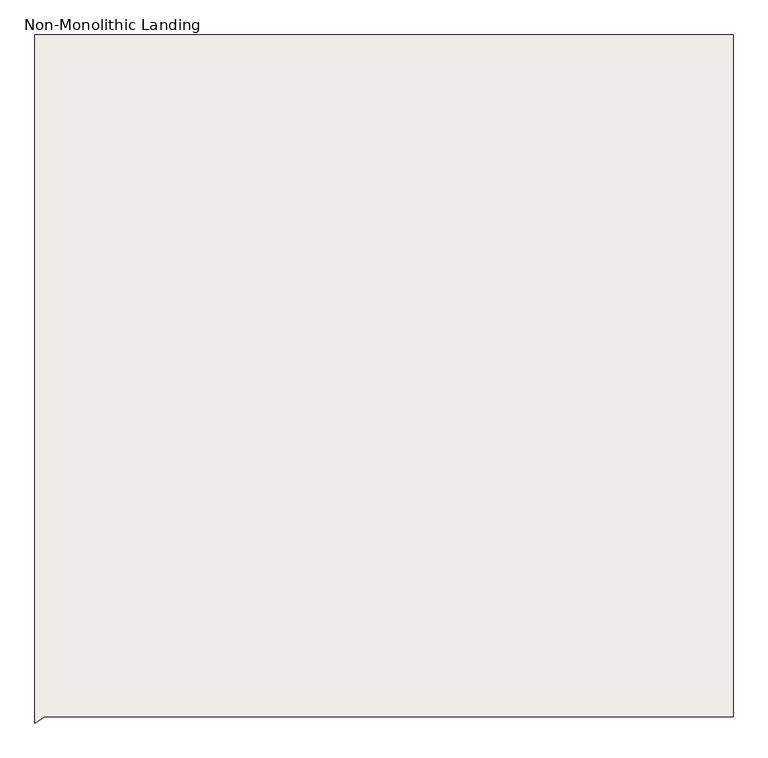
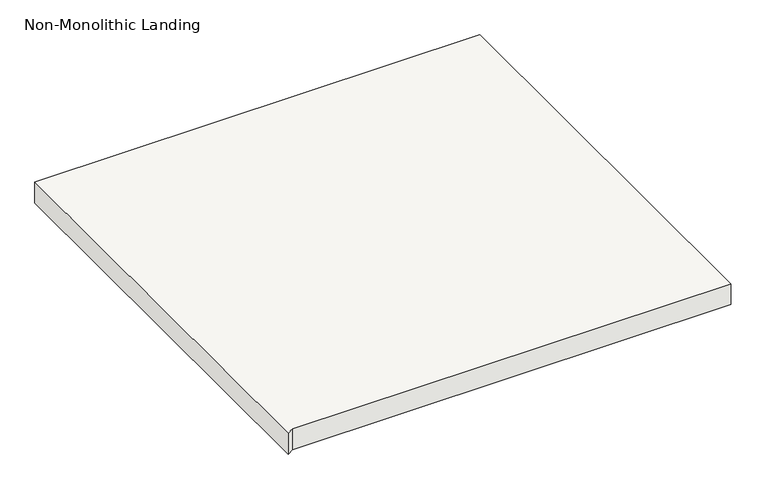
"""IFC4 building model written with IfcOpenShell, lengths in millimetres: slab geometry, Non-Monolithic Landing."""

from ifc_helpers import new_model, si_unit, frame, origin, place, context, project, spatial, polyline, outline, extrude, source, transform, mapped, element, save


def non_monolithic_landing_cef648f3(model_context):
    return source(origin(), model_context, "Body", "SweptSolid", [
        extrude(outline(polyline([(-10492.1794909, -1507.9618509), (-9477.5794909, -1507.9618509), (-9477.5794909, -2498.5618509), (-10477.6052721, -2498.5618509), (-10492.1794909, -2507.9876321), (-10492.1794909, -1507.9618509)])), frame((0.0, 0.0, 10869.0117647), z_axis=(0.0, 0.0, 1.0), x_axis=(1.0, 0.0, 0.0)), (0.0, 0.0, 1.0), 50.0),
    ])


if __name__ == "__main__":
    model = new_model("IFC4")
    model_context = context("Model", 3, world=origin())
    ifc_project = project(units=[si_unit("LENGTHUNIT", "METRE", prefix="MILLI")], contexts=[model_context])
    site = spatial("IfcSite", under=ifc_project)
    building = spatial("IfcBuilding", under=site)
    placement = place(None, origin())
    non_monolithic_landing_shape = non_monolithic_landing_cef648f3(model_context)
    element("IfcSlab", 1, ObjectType="Non-Monolithic Landing", at=placement, inside=building, context=model_context, shape_type="MappedRepresentation", body=[
        mapped(non_monolithic_landing_shape, transform((0.0, 0.0, 0.0), x_axis=(1.0, 0.0, 0.0), y_axis=(0.0, 1.0, 0.0), z_axis=(0.0, 0.0, 1.0))),
    ])
    save(model, "model.ifc")
